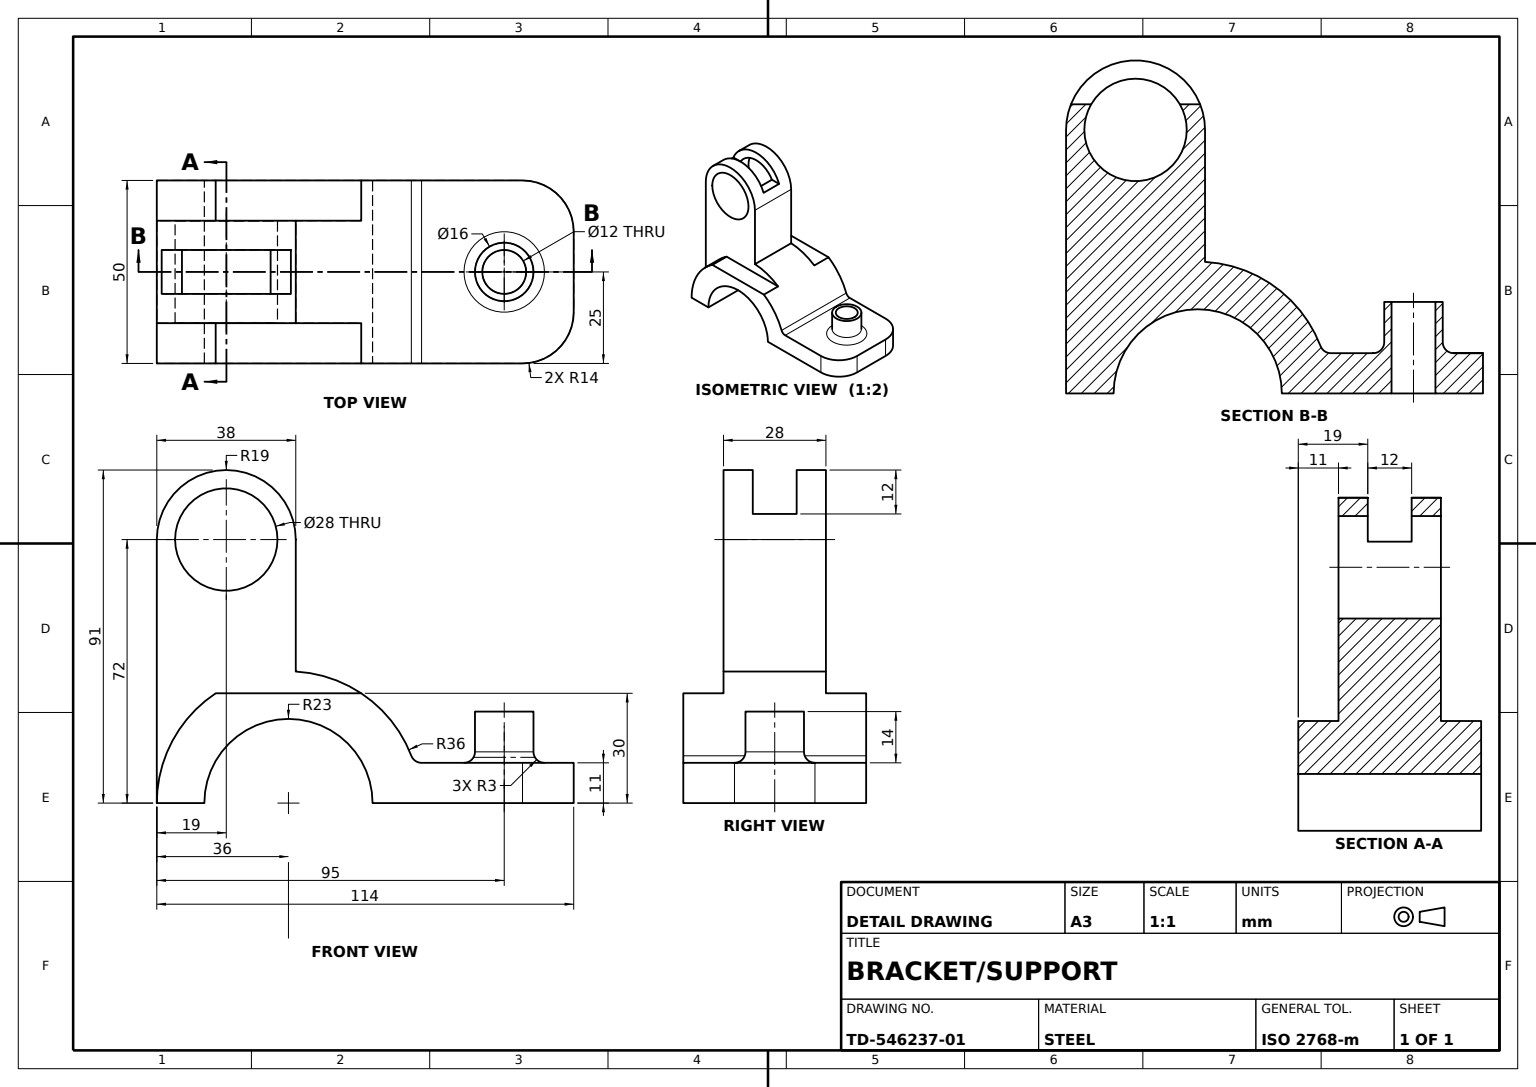
from build123d import *

# Parameters (mm, degrees)
BASE_SADDLE_DEPTH          = 25
BASE_CORNER_FILLET_R14_R   = 14
PIN_BOSS_SKETCH_R          = 8
PIVOT_PIN_BOSS_16_DEPTH    = 14
PIN_BOSS_BORE_SKETCH_R     = 6
PIN_BOSS_BORE_12_DEPTH     = 86.638776264
PIN_BOSS_ROOT_FILLET_R3_R  = 3
CLEVIS_UPRIGHT_DEPTH       = 14
EYE_BOSS_SKETCH_R          = 19
EYE_BOSS_DEPTH             = 14
EYE_BORE_SKETCH_R          = 14
EYE_BORE_28_DEPTH          = 127.039676293
SADDLE_START               = -11
SADDLE_CLEARANCE_CUT_DEPTH = 11
SADDLE_RELIEF_CUT_DEPTH    = 11
CLEVIS_SLOT_SKETCH_W       = 12
CLEVIS_SLOT_SKETCH_H       = 38
CLEVIS_SLOT_12_DEPTH       = 12


with BuildPart() as part:
    # Base Saddle Profile Sketch → Base Saddle (new, symmetric)
    with BuildSketch(Plane(origin=(0, 0, 0), x_dir=(0, 0, -1), z_dir=(1, 0, 0))):
        with BuildLine():
            Line((23, 0), (78, 0))
            Line((78, 0), (78, 11))
            Line((78, 11), (34.278273002, 11))
            ThreePointArc((34.278273002, 11), (-5.566963801, 35.566963801), (-36, 0))
            Line((-36, 0), (-23, 0))
            ThreePointArc((-23, 0), (0, 23), (23, 0))
        make_face()
    extrude(amount=BASE_SADDLE_DEPTH, both=True)

    # Base Corner Fillet R14
    base_corner_fillet_r14_edges = [part.edges().sort_by_distance(p)[0] for p in [
        (25, 5.5, -78),
        (-25, 5.5, -78),
    ]]
    fillet(base_corner_fillet_r14_edges, radius=BASE_CORNER_FILLET_R14_R)

    # Pin Boss Sketch → Pivot Pin Boss Ø16 (add)
    with BuildSketch(Plane(origin=(0, 11, 0), x_dir=(1, 0, 0), z_dir=(0, 1, 0))):
        with Locations(Location((0, 59, 0), (0, 0, 90))):
            Circle(PIN_BOSS_SKETCH_R)
    extrude(amount=PIVOT_PIN_BOSS_16_DEPTH)

    # Pin Boss Bore Sketch → Pin Boss Bore Ø12 (cut, through all)
    with BuildSketch(Plane(origin=(0, 25, 0), x_dir=(1, 0, 0), z_dir=(0, 1, 0))):
        with Locations(Location((0, 59, 0), (0, 0, 270))):
            Circle(PIN_BOSS_BORE_SKETCH_R)
    extrude(amount=-PIN_BOSS_BORE_12_DEPTH, mode=Mode.SUBTRACT)

    # Pin Boss Root Fillet R3
    pin_boss_root_fillet_r3_edges = [part.edges().sort_by_distance(p)[0] for p in [
        (0, 11, -34.278273002),
        (0, 11, -51),
    ]]
    fillet(pin_boss_root_fillet_r3_edges, radius=PIN_BOSS_ROOT_FILLET_R3_R)

    # Clevis Upright Sketch → Clevis Upright (add, symmetric)
    with BuildSketch(Plane(origin=(0, 0, 0), x_dir=(0, 0, -1), z_dir=(1, 0, 0))):
        with BuildLine():
            Line((-36, 0), (-36, 72))
            Line((-36, 72), (2, 72))
            Line((2, 72), (2, 35.944401511))
            ThreePointArc((2, 35.944401511), (-24.738633754, 26.153393661), (-36, 0))
        make_face()
    extrude(amount=CLEVIS_UPRIGHT_DEPTH, both=True)

    # Eye Boss Sketch → Eye Boss (add, symmetric)
    with BuildSketch(Plane(origin=(0, 0, 0), x_dir=(0, 0, -1), z_dir=(1, 0, 0))):
        with Locations((-17, 72)):
            Circle(EYE_BOSS_SKETCH_R)
    extrude(amount=EYE_BOSS_DEPTH, both=True)

    # Eye Bore Sketch → Eye Bore Ø28 (cut, through all)
    with BuildSketch(Plane.ZY.offset(14)):
        with Locations((17, 72)):
            Circle(EYE_BORE_SKETCH_R)
    extrude(amount=-EYE_BORE_28_DEPTH, mode=Mode.SUBTRACT)

    # Saddle Clearance Sketch → Saddle Clearance Cut (cut)
    with BuildSketch(Plane.ZY.offset(25).offset(SADDLE_START)):
        with BuildLine():
            Line((-19.899748742, 30), (19.899748742, 30))
            ThreePointArc((19.899748742, 30), (0, 36), (-19.899748742, 30))
        make_face()
    extrude(amount=SADDLE_CLEARANCE_CUT_DEPTH, mode=Mode.SUBTRACT)

    # Saddle Relief Sketch → Saddle Relief Cut (cut)
    with BuildSketch(Plane(origin=(25, 0, 0), x_dir=(0, 0, -1), z_dir=(1, 0, 0))):
        with BuildLine():
            Line((19.899748742, 30), (-19.899748742, 30))
            ThreePointArc((-19.899748742, 30), (0, 36), (19.899748742, 30))
        make_face()
    extrude(amount=-SADDLE_RELIEF_CUT_DEPTH, mode=Mode.SUBTRACT)

    # Clevis Slot Sketch → Clevis Slot 12 (cut)
    with BuildSketch(Plane(origin=(0, 91, 0), x_dir=(-1, 0, 0), z_dir=(0, -1, 0))):
        with Locations((0, -17)):
            Rectangle(CLEVIS_SLOT_SKETCH_W, CLEVIS_SLOT_SKETCH_H)
    extrude(amount=CLEVIS_SLOT_12_DEPTH, mode=Mode.SUBTRACT)


solid = part.part
